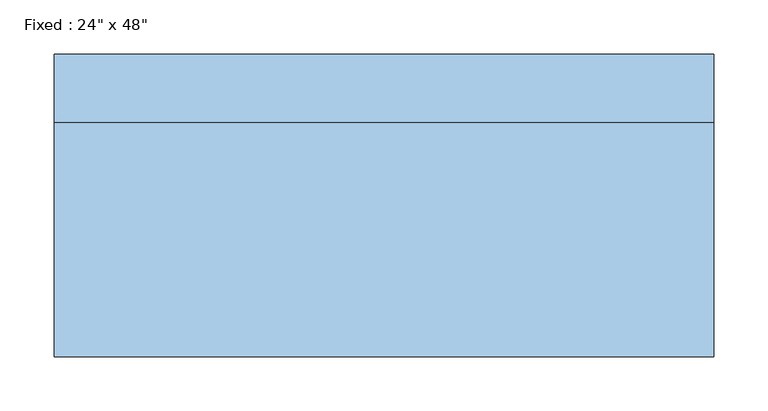
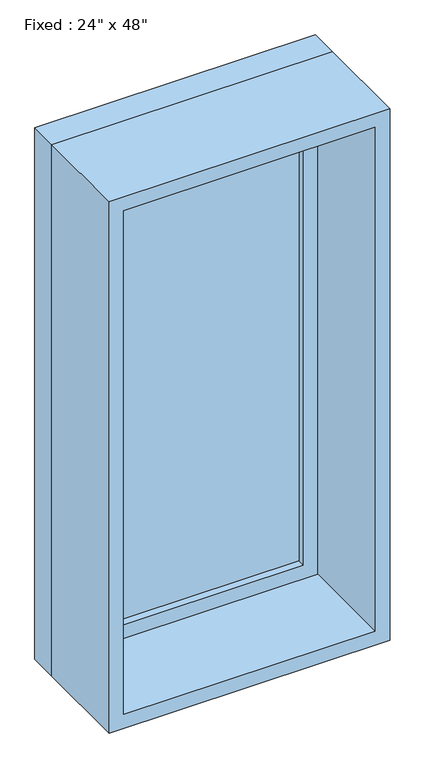
"""IFC4 building model written with IfcOpenShell, lengths in millimetres: window geometry."""

from ifc_helpers import new_model, si_unit, frame, origin, place, context, project, spatial, polyline, outline, extrude, source, transform, mapped, element, save


def window_dff46b58(model_context):
    return source(origin(), model_context, "Body", "SweptSolid", [
        extrude(outline(polyline([(203.2, 92.075), (-279.4, 92.075), (-279.4, 104.775), (203.2, 104.775), (203.2, 92.075)])), frame((0.0, 0.0, 977.9), z_axis=(0.0, 0.0, 1.0), x_axis=(1.0, 0.0, 0.0)), (0.0, 0.0, 1.0), 1092.2),
        extrude(outline(polyline([(2114.55, -323.85), (933.45, -323.85), (933.45, 247.65), (2114.55, 247.65), (2114.55, -323.85)]), holes=[polyline([(2070.1, -279.4), (2070.1, 203.2), (977.9, 203.2), (977.9, -279.4), (2070.1, -279.4)])]), frame((0.0, 76.2, 0.0), z_axis=(0.0, 1.0, 0.0), x_axis=(0.0, 0.0, 1.0)), (0.0, 0.0, 1.0), 44.45),
        extrude(outline(polyline([(2133.6, -342.9), (914.4, -342.9), (914.4, 266.7), (2133.6, 266.7), (2133.6, -342.9)]), holes=[polyline([(2101.85, -311.15), (2101.85, 234.95), (946.15, 234.95), (946.15, -311.15), (2101.85, -311.15)])]), frame((0.0, -139.7, 0.0), z_axis=(0.0, 1.0, 0.0), x_axis=(0.0, 0.0, 1.0)), (0.0, 0.0, 1.0), 215.9),
        extrude(outline(polyline([(2133.6, 266.7), (2133.6, -342.9), (914.4, -342.9), (914.4, 266.7), (2133.6, 266.7)]), holes=[polyline([(2114.55, 247.65), (933.45, 247.65), (933.45, -323.85), (2114.55, -323.85), (2114.55, 247.65)])]), frame((0.0, 76.2, 0.0), z_axis=(0.0, 1.0, 0.0), x_axis=(0.0, 0.0, 1.0)), (0.0, 0.0, 1.0), 63.5),
    ])


if __name__ == "__main__":
    model = new_model("IFC4")
    model_context = context("Model", 3, world=origin())
    ifc_project = project(units=[si_unit("LENGTHUNIT", "METRE", prefix="MILLI")], contexts=[model_context])
    site = spatial("IfcSite", under=ifc_project)
    building = spatial("IfcBuilding", under=site)
    placement = place(None, origin())
    window_shape = window_dff46b58(model_context)
    element("IfcWindow", 1, ObjectType="Fixed : 24\" x 48\"", at=placement, inside=building, context=model_context, shape_type="MappedRepresentation", body=[
        mapped(window_shape, transform((0.0, 0.0, 0.0), x_axis=(1.0, 0.0, 0.0), y_axis=(0.0, 1.0, 0.0), z_axis=(0.0, 0.0, 1.0))),
    ])
    save(model, "model.ifc")

# Revit data of these elements
# Type "Fixed : 24\" x 48\""
#   Type Mark = "2"
#   Construction Type Id = "GSP4R"
#   Assembly Code = "B2020100"
#   Analytic Construction = "1/8 in Pilkington single glazing"
#   Visual Light Transmittance = 0.9
#   Solar Heat Gain Coefficient = 0.78
#   Heat Transfer Coefficient (U) = 0.6496 BTU/(h·ft²·°F)
#   Height = 4' - 0"
#   Default Sill Height = 3' - 0"
#   Width = 2' - 0"
#   Window Inset = 0' - 0 3/4"
#   Define Thermal Properties by = 1
#   Define Thermal Properties by = 1
#   Glass Pane Material = Glass
#   Sash Material = Sash
#   Wall Closure = (empty or 0)
# Element 1 (IfcWindow, "Fixed : 24\" x 48\"")
#   Materials on its faces: "Sash", "Glass"
# Materials
#   "Glass": class "Glass", colour RGB 0 128 192, transparency 0.75, Description = "Soda Lime Glass", Cost = 0
#   "Sash": class "Wood", colour RGB 224 178 126, transparency 0, Cost = 0
